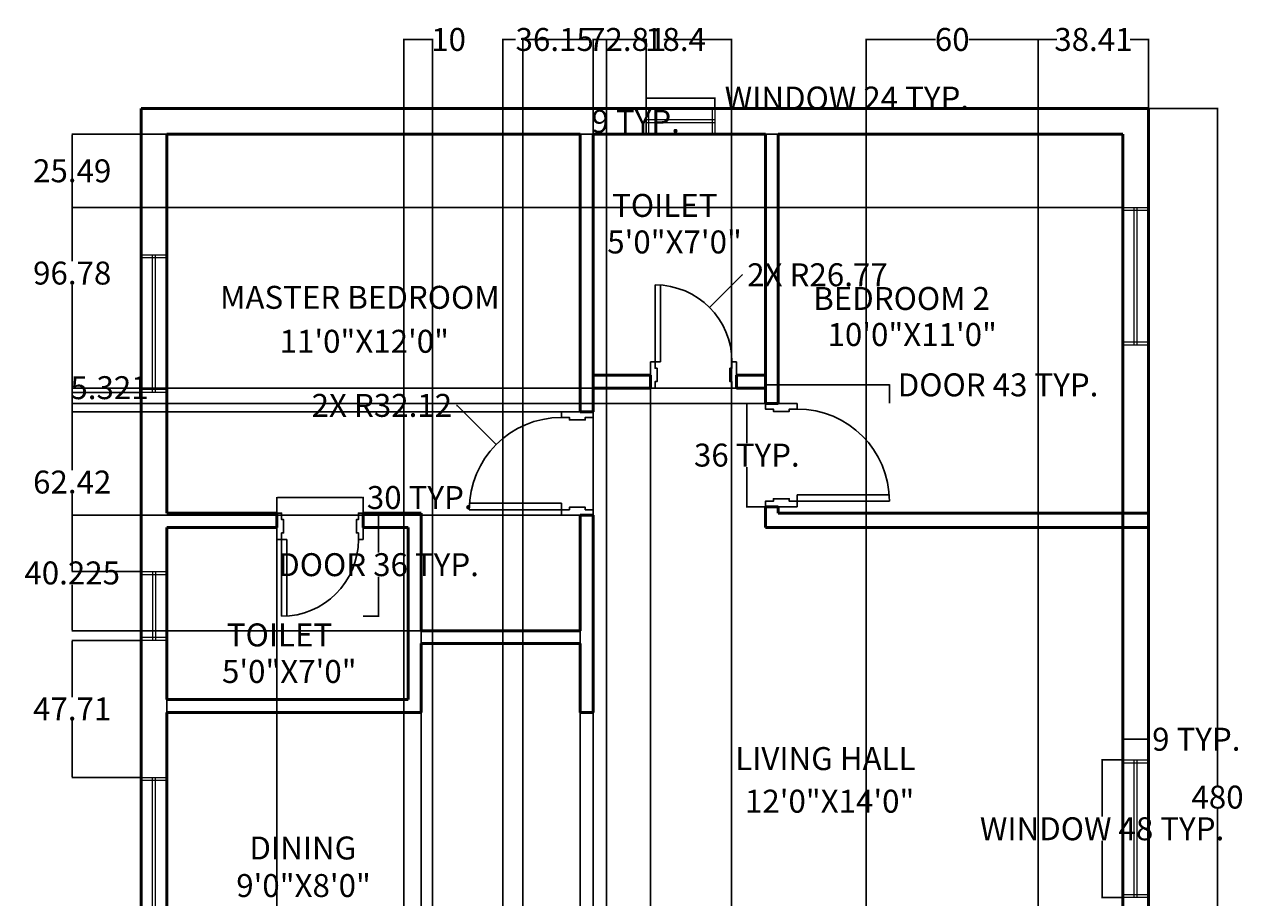
# Model space of a CAD drawing. Units: inches. Extents: x 16123781 to 16124206, y 158262361 to 158262900.
# Tile 2 of 2: x 16123781 to 16124206, y 158262596 to 158262900. Entities that reach past the tile are written whole.
import ezdxf

# ---------------------------------------------------------------- set-up
doc = ezdxf.new("R2010")
doc.units = ezdxf.units.IN
for name, color, linetype, lineweight in [('A-ANNO-DIMS', 2, 'Continuous', 18), ('A-AREA-IDEN', 7, 'Continuous', 25), ('A-Door', 150, 'Continuous', 25), ('wall', 130, 'Continuous', 50), ('window', 80, 'Continuous', 18)]:
    doc.layers.add(name, color=color, linetype=linetype, lineweight=lineweight)
doc.styles.get("Standard").update_dxf_attribs({"font": 'arial.ttf', "height": 8})
doc.dimstyles.get("Standard").update_dxf_attribs({"dimtxt": 0.18, "dimasz": 0.18, "dimexe": 0.18, "dimexo": 0.0625, "dimgap": 0.09, "dimtad": 0, "dimtih": 1, "dimtoh": 1, "dimdec": 4, "dimzin": 0, "dimdsep": 46, "dimtxsty": 'Standard', "dimcen": 0.09, "dimadec": 0, "dimazin": 0, "dimtfac": 1, "dimtdec": 4, "dimtofl": 0, "dimtmove": 0, "dimatfit": 3, "dimfxl": 1, "dimtolj": 1, "dimtzin": 0, "dimarcsym": 0})

# ---------------------------------------------------------------- blocks, each defined once
blk = doc.blocks.new('AP0B01')
blk.add_line((75, 100), (75, 678.7))
blk.add_lwpolyline([(35, 100), (35, 680, -0.449922)], format="xyb")
for points in [[(0, 100), (0, -100), (35, -100), (35, -50), (50, -50), (50, 50), (35, 50), (35, 100)], [(650, 100), (650, -100), (615, -100), (615, -50), (600, -50), (600, 50), (615, 50), (615, 100)]]:
    blk.add_lwpolyline(points, close=True)
blk.add_lwpolyline([(35, 100), (75, 100)])
blk.add_arc((35, 100), 580, 0, 90)
blk = doc.blocks.new('WIN-48IN')
for p, q in [((0, 0), (0, 48)), ((0, 48), (9, 48)), ((0, 47), (9, 47)), ((4, 0), (4, 48)), ((5, 0), (5, 48)), ((9, 48), (9, 0)), ((9, 1), (0, 1)), ((9, 0), (0, 0))]:
    blk.add_line(p, q)
blk = doc.blocks.new('WIN-24IN')
for p, q in [((0, 9), (24, 9)), ((0, 0), (0, 9)), ((1, 0), (1, 9)), ((23, 9), (23, 0)), ((24, 9), (24, 0)), ((24, 5), (0, 5)), ((24, 4), (0, 4)), ((24, 0), (0, 0))]:
    blk.add_line(p, q)
blk = doc.blocks.new('*D7')
at = {"layer": 'A-ANNO-DIMS', "color": 0, "lineweight": -2, "transparency": 16777216}
for p, q in [((16123899.14, 158262729.56), (16123904.65, 158262729.56)), ((16123904.47, 158262729.38), (16123904.47, 158262715.79)), ((16123904.47, 158262693.74), (16123904.47, 158262707.33)), ((16123899.14, 158262693.56), (16123904.65, 158262693.56))]:
    blk.add_line(p, q, dxfattribs=at)
at = {"layer": 'A-ANNO-DIMS', "color": 0, "transparency": 16777216}
for points in [[(16123904.44, 158262729.38), (16123904.5, 158262729.38), (16123904.47, 158262729.56)], [(16123904.44, 158262693.74), (16123904.5, 158262693.74), (16123904.47, 158262693.56)]]:
    blk.add_solid(points, dxfattribs=at)
at = {"layer": 'Defpoints', "color": 0, "transparency": 16777216}
for p in [(16123899.07, 158262729.56), (16123899.07, 158262693.56), (16123904.47, 158262693.56)]:
    blk.add_point(p, dxfattribs=at)
at = {"layer": 'A-ANNO-DIMS', "color": 0, "transparency": 16777216, "insert": (16123904.47, 158262711.56), "char_height": 8, "attachment_point": 5}
blk.add_mtext('\\A1;DOOR 36 TYP.', dxfattribs=at)
blk = doc.blocks.new('*D8')
at = {"layer": 'A-ANNO-DIMS', "color": 0, "lineweight": -2, "transparency": 16777216}
for p, q in [((16123869.07, 158262729.63), (16123869.07, 158262735.14)), ((16123869.25, 158262734.96), (16123898.89, 158262734.96)), ((16123899.07, 158262729.63), (16123899.07, 158262735.14)), ((16123899.07, 158262734.96), (16123899.25, 158262734.96))]:
    blk.add_line(p, q, dxfattribs=at)
at = {"layer": 'A-ANNO-DIMS', "color": 0, "transparency": 16777216}
for points in [[(16123869.25, 158262734.99), (16123869.25, 158262734.93), (16123869.07, 158262734.96)], [(16123898.89, 158262734.99), (16123898.89, 158262734.93), (16123899.07, 158262734.96)]]:
    blk.add_solid(points, dxfattribs=at)
at = {"layer": 'Defpoints', "color": 0, "transparency": 16777216}
for p in [(16123899.07, 158262734.96), (16123869.07, 158262729.56), (16123899.07, 158262729.56)]:
    blk.add_point(p, dxfattribs=at)
at = {"layer": 'A-ANNO-DIMS', "color": 0, "transparency": 16777216, "insert": (16123918.81, 158262734.96), "char_height": 8, "attachment_point": 5}
blk.add_mtext('\\A1;30 TYP.', dxfattribs=at)
blk = doc.blocks.new('*D9')
at = {"layer": 'A-ANNO-DIMS', "color": 0, "lineweight": -2, "transparency": 16777216}
for p, q in [((16124039.26, 158262767.8), (16124039.26, 158262774.4)), ((16124082.46, 158262767.8), (16124082.46, 158262774.4)), ((16124039.44, 158262774.22), (16124082.28, 158262774.22)), ((16124082.46, 158262774.22), (16124082.64, 158262774.22))]:
    blk.add_line(p, q, dxfattribs=at)
at = {"layer": 'A-ANNO-DIMS', "color": 0, "transparency": 16777216}
for points in [[(16124039.44, 158262774.25), (16124039.44, 158262774.19), (16124039.26, 158262774.22)], [(16124082.28, 158262774.25), (16124082.28, 158262774.19), (16124082.46, 158262774.22)]]:
    blk.add_solid(points, dxfattribs=at)
at = {"layer": 'Defpoints', "color": 0, "transparency": 16777216}
for p in [(16124082.46, 158262774.22), (16124039.26, 158262767.74), (16124082.46, 158262767.74)]:
    blk.add_point(p, dxfattribs=at)
at = {"layer": 'A-ANNO-DIMS', "color": 0, "transparency": 16777216, "insert": (16124120.32, 158262774.22), "char_height": 8, "attachment_point": 5}
blk.add_mtext('\\A1;DOOR 43 TYP.', dxfattribs=at)
blk = doc.blocks.new('*D10')
at = {"layer": 'A-ANNO-DIMS', "color": 0, "lineweight": -2, "transparency": 16777216}
for p, q in [((16124039.2, 158262767.74), (16124032.6, 158262767.74)), ((16124032.78, 158262767.56), (16124032.78, 158262753.92)), ((16124032.78, 158262731.92), (16124032.78, 158262745.56)), ((16124039.2, 158262731.74), (16124032.6, 158262731.74))]:
    blk.add_line(p, q, dxfattribs=at)
at = {"layer": 'A-ANNO-DIMS', "color": 0, "transparency": 16777216}
for points in [[(16124032.75, 158262767.56), (16124032.81, 158262767.56), (16124032.78, 158262767.74)], [(16124032.75, 158262731.92), (16124032.81, 158262731.92), (16124032.78, 158262731.74)]]:
    blk.add_solid(points, dxfattribs=at)
at = {"layer": 'Defpoints', "color": 0, "transparency": 16777216}
for p in [(16124032.78, 158262767.74), (16124039.26, 158262767.74), (16124039.26, 158262731.74)]:
    blk.add_point(p, dxfattribs=at)
at = {"layer": 'A-ANNO-DIMS', "color": 0, "transparency": 16777216, "insert": (16124032.78, 158262749.74), "char_height": 8, "attachment_point": 5}
blk.add_mtext('\\A1;36 TYP.', dxfattribs=at)
blk = doc.blocks.new('*D11')
at = {"layer": 'A-ANNO-DIMS', "color": 0, "lineweight": -2, "transparency": 16777216}
for p, q in [((16124163.7, 158262643.53), (16124156.38, 158262643.53)), ((16124156.56, 158262643.35), (16124156.56, 158262623.76)), ((16124156.56, 158262595.71), (16124156.56, 158262615.31)), ((16124163.7, 158262595.53), (16124156.38, 158262595.53))]:
    blk.add_line(p, q, dxfattribs=at)
at = {"layer": 'A-ANNO-DIMS', "color": 0, "transparency": 16777216}
for points in [[(16124156.53, 158262643.35), (16124156.59, 158262643.35), (16124156.56, 158262643.53)], [(16124156.53, 158262595.71), (16124156.59, 158262595.71), (16124156.56, 158262595.53)]]:
    blk.add_solid(points, dxfattribs=at)
at = {"layer": 'Defpoints', "color": 0, "transparency": 16777216}
for p in [(16124156.56, 158262643.53), (16124163.76, 158262643.53), (16124163.76, 158262595.53)]:
    blk.add_point(p, dxfattribs=at)
at = {"layer": 'A-ANNO-DIMS', "color": 0, "transparency": 16777216, "insert": (16124156.56, 158262619.53), "char_height": 8, "attachment_point": 5}
blk.add_mtext('\\A1;WINDOW 48 TYP.', dxfattribs=at)
blk = doc.blocks.new('*D12')
at = {"layer": 'A-ANNO-DIMS', "color": 0, "lineweight": -2, "transparency": 16777216}
for p, q in [((16124163.76, 158262643.6), (16124163.76, 158262650.91)), ((16124163.94, 158262650.73), (16124172.58, 158262650.73)), ((16124172.76, 158262643.6), (16124172.76, 158262650.91)), ((16124172.76, 158262650.73), (16124172.94, 158262650.73))]:
    blk.add_line(p, q, dxfattribs=at)
at = {"layer": 'A-ANNO-DIMS', "color": 0, "transparency": 16777216}
for points in [[(16124163.94, 158262650.76), (16124163.94, 158262650.7), (16124163.76, 158262650.73)], [(16124172.58, 158262650.76), (16124172.58, 158262650.7), (16124172.76, 158262650.73)]]:
    blk.add_solid(points, dxfattribs=at)
at = {"layer": 'Defpoints', "color": 0, "transparency": 16777216}
for p in [(16124172.76, 158262650.73), (16124163.76, 158262643.53), (16124172.76, 158262643.53)]:
    blk.add_point(p, dxfattribs=at)
at = {"layer": 'A-ANNO-DIMS', "color": 0, "transparency": 16777216, "insert": (16124189.39, 158262650.73), "char_height": 8, "attachment_point": 5}
blk.add_mtext('\\A1;9 TYP.', dxfattribs=at)
blk = doc.blocks.new('*D13')
at = {"layer": 'A-ANNO-DIMS', "color": 0, "lineweight": -2, "transparency": 16777216}
for p, q in [((16123997.66, 158262870.63), (16123997.66, 158262874.34)), ((16123997.84, 158262874.16), (16124021.48, 158262874.16)), ((16124021.66, 158262870.63), (16124021.66, 158262874.34)), ((16124021.66, 158262874.16), (16124021.84, 158262874.16))]:
    blk.add_line(p, q, dxfattribs=at)
at = {"layer": 'A-ANNO-DIMS', "color": 0, "transparency": 16777216}
for points in [[(16123997.84, 158262874.19), (16123997.84, 158262874.13), (16123997.66, 158262874.16)], [(16124021.48, 158262874.19), (16124021.48, 158262874.13), (16124021.66, 158262874.16)]]:
    blk.add_solid(points, dxfattribs=at)
at = {"layer": 'Defpoints', "color": 0, "transparency": 16777216}
for p in [(16124021.66, 158262874.16), (16123997.66, 158262870.56), (16124021.66, 158262870.56)]:
    blk.add_point(p, dxfattribs=at)
at = {"layer": 'A-ANNO-DIMS', "color": 0, "transparency": 16777216, "insert": (16124067.64, 158262874.16), "char_height": 8, "attachment_point": 5}
blk.add_mtext('\\A1;WINDOW 24 TYP.', dxfattribs=at)
blk = doc.blocks.new('*D14')
at = {"layer": 'A-ANNO-DIMS', "color": 0, "lineweight": -2, "transparency": 16777216}
for p, q in [((16123997.6, 158262870.56), (16123993.88, 158262870.56)), ((16123994.06, 158262870.38), (16123994.06, 158262870.24)), ((16123997.6, 158262861.56), (16123993.88, 158262861.56)), ((16123994.06, 158262861.74), (16123994.06, 158262861.89))]:
    blk.add_line(p, q, dxfattribs=at)
at = {"layer": 'A-ANNO-DIMS', "color": 0, "transparency": 16777216}
for points in [[(16123994.03, 158262870.38), (16123994.09, 158262870.38), (16123994.06, 158262870.56)], [(16123994.03, 158262861.74), (16123994.09, 158262861.74), (16123994.06, 158262861.56)]]:
    blk.add_solid(points, dxfattribs=at)
at = {"layer": 'Defpoints', "color": 0, "transparency": 16777216}
for p in [(16123994.06, 158262870.56), (16123997.66, 158262870.56), (16123997.66, 158262861.56)]:
    blk.add_point(p, dxfattribs=at)
at = {"layer": 'A-ANNO-DIMS', "color": 0, "transparency": 16777216, "insert": (16123994.06, 158262866.06), "char_height": 8, "attachment_point": 5}
blk.add_mtext('\\A1;9 TYP.', dxfattribs=at)
blk = doc.blocks.new('*D18')
at = {"layer": 'A-ANNO-DIMS', "color": 0, "lineweight": -2, "transparency": 16777216}
for p, q in [((16124172.82, 158262870.56), (16124196.97, 158262870.56)), ((16124196.79, 158262870.38), (16124196.79, 158262634.74)), ((16124196.79, 158262390.74), (16124196.79, 158262626.39)), ((16124172.82, 158262390.56), (16124196.97, 158262390.56))]:
    blk.add_line(p, q, dxfattribs=at)
at = {"layer": 'A-ANNO-DIMS', "color": 0, "transparency": 16777216}
for points in [[(16124196.76, 158262870.38), (16124196.82, 158262870.38), (16124196.79, 158262870.56)], [(16124196.76, 158262390.74), (16124196.82, 158262390.74), (16124196.79, 158262390.56)]]:
    blk.add_solid(points, dxfattribs=at)
at = {"layer": 'Defpoints', "color": 0, "transparency": 16777216}
for p in [(16124172.76, 158262870.56), (16124196.79, 158262870.56), (16124172.76, 158262390.56)]:
    blk.add_point(p, dxfattribs=at)
at = {"layer": 'A-ANNO-DIMS', "color": 0, "transparency": 16777216, "insert": (16124196.79, 158262630.56), "char_height": 8, "attachment_point": 5}
blk.add_mtext('\\A1;480', dxfattribs=at)
blk = doc.blocks.new('*D19')
at = {"layer": 'A-ANNO-DIMS', "color": 0, "lineweight": -2, "transparency": 16777216}
for p, q in [((16124074.35, 158262390.63), (16124074.35, 158262894.77)), ((16124074.53, 158262894.59), (16124098.52, 158262894.59)), ((16124134.17, 158262894.59), (16124110.18, 158262894.59)), ((16124134.35, 158262390.63), (16124134.35, 158262894.77))]:
    blk.add_line(p, q, dxfattribs=at)
at = {"layer": 'A-ANNO-DIMS', "color": 0, "transparency": 16777216}
for points in [[(16124074.53, 158262894.62), (16124074.53, 158262894.56), (16124074.35, 158262894.59)], [(16124134.17, 158262894.62), (16124134.17, 158262894.56), (16124134.35, 158262894.59)]]:
    blk.add_solid(points, dxfattribs=at)
at = {"layer": 'Defpoints', "color": 0, "transparency": 16777216}
for p in [(16124134.35, 158262894.59), (16124074.35, 158262390.56), (16124134.35, 158262390.56)]:
    blk.add_point(p, dxfattribs=at)
at = {"layer": 'A-ANNO-DIMS', "color": 0, "transparency": 16777216, "insert": (16124104.35, 158262894.59), "char_height": 8, "attachment_point": 5}
blk.add_mtext('\\A1;60', dxfattribs=at)
blk = doc.blocks.new('*D20')
at = {"layer": 'A-ANNO-DIMS', "color": 0, "lineweight": -2, "transparency": 16777216}
for p, q in [((16124134.35, 158262390.63), (16124134.35, 158262894.77)), ((16124134.53, 158262894.59), (16124140.74, 158262894.59)), ((16124172.58, 158262894.59), (16124166.37, 158262894.59)), ((16124172.76, 158262390.63), (16124172.76, 158262894.77))]:
    blk.add_line(p, q, dxfattribs=at)
at = {"layer": 'A-ANNO-DIMS', "color": 0, "transparency": 16777216}
for points in [[(16124134.53, 158262894.62), (16124134.53, 158262894.56), (16124134.35, 158262894.59)], [(16124172.58, 158262894.62), (16124172.58, 158262894.56), (16124172.76, 158262894.59)]]:
    blk.add_solid(points, dxfattribs=at)
at = {"layer": 'Defpoints', "color": 0, "transparency": 16777216}
for p in [(16124172.76, 158262894.59), (16124134.35, 158262390.56), (16124172.76, 158262390.56)]:
    blk.add_point(p, dxfattribs=at)
at = {"layer": 'A-ANNO-DIMS', "color": 0, "transparency": 16777216, "insert": (16124153.55, 158262894.59), "char_height": 8, "attachment_point": 5}
blk.add_mtext('\\A1;38.41', dxfattribs=at)
blk = doc.blocks.new('*D23')
at = {"layer": 'A-ANNO-DIMS', "color": 0, "lineweight": -2, "transparency": 16777216}
for p, q in [((16123947.76, 158262503.13), (16123947.76, 158262894.77)), ((16123947.94, 158262894.59), (16123952.22, 158262894.59)), ((16123983.73, 158262894.59), (16123979.45, 158262894.59)), ((16123983.91, 158262503.13), (16123983.91, 158262894.77))]:
    blk.add_line(p, q, dxfattribs=at)
at = {"layer": 'A-ANNO-DIMS', "color": 0, "transparency": 16777216}
for points in [[(16123947.94, 158262894.62), (16123947.94, 158262894.56), (16123947.76, 158262894.59)], [(16123983.73, 158262894.62), (16123983.73, 158262894.56), (16123983.91, 158262894.59)]]:
    blk.add_solid(points, dxfattribs=at)
at = {"layer": 'Defpoints', "color": 0, "transparency": 16777216}
for p in [(16123983.91, 158262894.59), (16123947.76, 158262503.06), (16123983.91, 158262503.06)]:
    blk.add_point(p, dxfattribs=at)
at = {"layer": 'A-ANNO-DIMS', "color": 0, "transparency": 16777216, "insert": (16123965.84, 158262894.59), "char_height": 8, "attachment_point": 5}
blk.add_mtext('\\A1;36.15', dxfattribs=at)
blk = doc.blocks.new('*D29')
at = {"layer": 'A-ANNO-DIMS', "color": 0, "lineweight": -2, "transparency": 16777216}
for p, q in [((16123821.7, 158262685.14), (16123797.55, 158262685.14)), ((16123797.73, 158262684.96), (16123797.73, 158262665.39)), ((16123797.73, 158262637.61), (16123797.73, 158262657.18)), ((16123821.7, 158262637.43), (16123797.55, 158262637.43))]:
    blk.add_line(p, q, dxfattribs=at)
at = {"layer": 'A-ANNO-DIMS', "color": 0, "transparency": 16777216}
for points in [[(16123797.7, 158262684.96), (16123797.76, 158262684.96), (16123797.73, 158262685.14)], [(16123797.7, 158262637.61), (16123797.76, 158262637.61), (16123797.73, 158262637.43)]]:
    blk.add_solid(points, dxfattribs=at)
at = {"layer": 'Defpoints', "color": 0, "transparency": 16777216}
for p in [(16123797.73, 158262685.14), (16123821.76, 158262685.14), (16123821.76, 158262637.43)]:
    blk.add_point(p, dxfattribs=at)
at = {"layer": 'A-ANNO-DIMS', "color": 0, "transparency": 16777216, "insert": (16123797.73, 158262661.29), "char_height": 8, "attachment_point": 5}
blk.add_mtext('\\A1;47.71', dxfattribs=at)
blk = doc.blocks.new('*D30')
at = {"layer": 'A-ANNO-DIMS', "color": 0, "lineweight": -2, "transparency": 16777216}
for p, q in [((16123821.7, 158262771.56), (16123797.55, 158262771.56)), ((16123797.73, 158262771.38), (16123797.73, 158262744.53)), ((16123797.73, 158262709.32), (16123797.73, 158262736.18)), ((16123821.7, 158262709.14), (16123797.55, 158262709.14))]:
    blk.add_line(p, q, dxfattribs=at)
at = {"layer": 'A-ANNO-DIMS', "color": 0, "transparency": 16777216}
for points in [[(16123797.7, 158262771.38), (16123797.76, 158262771.38), (16123797.73, 158262771.56)], [(16123797.7, 158262709.32), (16123797.76, 158262709.32), (16123797.73, 158262709.14)]]:
    blk.add_solid(points, dxfattribs=at)
at = {"layer": 'Defpoints', "color": 0, "transparency": 16777216}
for p in [(16123797.73, 158262771.56), (16123821.76, 158262771.56), (16123821.76, 158262709.14)]:
    blk.add_point(p, dxfattribs=at)
at = {"layer": 'A-ANNO-DIMS', "color": 0, "transparency": 16777216, "insert": (16123797.73, 158262740.35), "char_height": 8, "attachment_point": 5}
blk.add_mtext('\\A1;62.42', dxfattribs=at)
blk = doc.blocks.new('*D32')
at = {"layer": 'A-ANNO-DIMS', "color": 0, "lineweight": -2, "transparency": 16777216}
for p, q in [((16124163.7, 158262861.56), (16123797.55, 158262861.56)), ((16123797.73, 158262861.38), (16123797.73, 158262852.99)), ((16123797.73, 158262836.25), (16123797.73, 158262844.64)), ((16124163.7, 158262836.07), (16123797.55, 158262836.07))]:
    blk.add_line(p, q, dxfattribs=at)
at = {"layer": 'A-ANNO-DIMS', "color": 0, "transparency": 16777216}
for points in [[(16123797.7, 158262861.38), (16123797.76, 158262861.38), (16123797.73, 158262861.56)], [(16123797.7, 158262836.25), (16123797.76, 158262836.25), (16123797.73, 158262836.07)]]:
    blk.add_solid(points, dxfattribs=at)
at = {"layer": 'Defpoints', "color": 0, "transparency": 16777216}
for p in [(16123797.73, 158262861.56), (16124163.76, 158262861.56), (16124163.76, 158262836.07)]:
    blk.add_point(p, dxfattribs=at)
at = {"layer": 'A-ANNO-DIMS', "color": 0, "transparency": 16777216, "insert": (16123797.73, 158262848.82), "char_height": 8, "attachment_point": 5}
blk.add_mtext('\\A1;25.49', dxfattribs=at)
blk = doc.blocks.new('*D33')
at = {"layer": 'A-ANNO-DIMS', "color": 0, "lineweight": -2, "transparency": 16777216}
for p, q in [((16123979.26, 158262861.63), (16123979.26, 158262894.77)), ((16123979.44, 158262894.59), (16123997.48, 158262894.59)), ((16123997.66, 158262861.63), (16123997.66, 158262894.77)), ((16123997.66, 158262894.59), (16123997.84, 158262894.59))]:
    blk.add_line(p, q, dxfattribs=at)
at = {"layer": 'A-ANNO-DIMS', "color": 0, "transparency": 16777216}
for points in [[(16123979.44, 158262894.62), (16123979.44, 158262894.56), (16123979.26, 158262894.59)], [(16123997.48, 158262894.62), (16123997.48, 158262894.56), (16123997.66, 158262894.59)]]:
    blk.add_solid(points, dxfattribs=at)
at = {"layer": 'Defpoints', "color": 0, "transparency": 16777216}
for p in [(16123997.66, 158262894.59), (16123979.26, 158262861.56), (16123997.66, 158262861.56)]:
    blk.add_point(p, dxfattribs=at)
at = {"layer": 'A-ANNO-DIMS', "color": 0, "transparency": 16777216, "insert": (16124007.93, 158262894.59), "char_height": 8, "attachment_point": 5}
blk.add_mtext('\\A1;18.4', dxfattribs=at)
blk = doc.blocks.new('*D35')
at = {"layer": 'A-ANNO-DIMS', "color": 0, "lineweight": -2, "transparency": 16777216}
for p, q in [((16123913.26, 158262484.13), (16123913.26, 158262894.77)), ((16123913.44, 158262894.59), (16123923.08, 158262894.59)), ((16123923.26, 158262484.13), (16123923.26, 158262894.77)), ((16123923.26, 158262894.59), (16123923.44, 158262894.59))]:
    blk.add_line(p, q, dxfattribs=at)
at = {"layer": 'A-ANNO-DIMS', "color": 0, "transparency": 16777216}
for points in [[(16123913.44, 158262894.62), (16123913.44, 158262894.56), (16123913.26, 158262894.59)], [(16123923.08, 158262894.62), (16123923.08, 158262894.56), (16123923.26, 158262894.59)]]:
    blk.add_solid(points, dxfattribs=at)
at = {"layer": 'Defpoints', "color": 0, "transparency": 16777216}
for p in [(16123923.26, 158262894.59), (16123913.26, 158262484.06), (16123923.26, 158262484.06)]:
    blk.add_point(p, dxfattribs=at)
at = {"layer": 'A-ANNO-DIMS', "color": 0, "transparency": 16777216, "insert": (16123928.87, 158262894.59), "char_height": 8, "attachment_point": 5}
blk.add_mtext('\\A1;10', dxfattribs=at)
blk = doc.blocks.new('*D36')
at = {"layer": 'A-ANNO-DIMS', "color": 0, "lineweight": -2, "transparency": 16777216}
for p, q in [((16123954.69, 158262552.13), (16123954.69, 158262894.77)), ((16123954.87, 158262894.59), (16123978.31, 158262894.59)), ((16124027.32, 158262894.59), (16124003.88, 158262894.59)), ((16124027.5, 158262552.13), (16124027.5, 158262894.77))]:
    blk.add_line(p, q, dxfattribs=at)
at = {"layer": 'A-ANNO-DIMS', "color": 0, "transparency": 16777216}
for points in [[(16123954.87, 158262894.62), (16123954.87, 158262894.56), (16123954.69, 158262894.59)], [(16124027.32, 158262894.62), (16124027.32, 158262894.56), (16124027.5, 158262894.59)]]:
    blk.add_solid(points, dxfattribs=at)
at = {"layer": 'Defpoints', "color": 0, "transparency": 16777216}
for p in [(16124027.5, 158262894.59), (16123954.69, 158262552.06), (16124027.5, 158262552.06)]:
    blk.add_point(p, dxfattribs=at)
at = {"layer": 'A-ANNO-DIMS', "color": 0, "transparency": 16777216, "insert": (16123991.1, 158262894.59), "char_height": 8, "attachment_point": 5}
blk.add_mtext('\\A1;72.81', dxfattribs=at)
blk = doc.blocks.new('*D37')
at = {"layer": 'A-ANNO-DIMS', "color": 0, "lineweight": -2, "transparency": 16777216}
for p, q in [((16123919.260748, 158262688.500323), (16123919.260748, 158262366.352823)), ((16123974.760748, 158262688.500323), (16123974.760748, 158262366.352823)), ((16123919.440748, 158262366.532823), (16123936.500557, 158262366.532823)), ((16123974.580748, 158262366.532823), (16123957.520939, 158262366.532823))]:
    blk.add_line(p, q, dxfattribs=at)
at = {"layer": 'A-ANNO-DIMS', "color": 0, "transparency": 16777216}
for points in [[(16123919.440748, 158262366.562823), (16123919.440748, 158262366.502823), (16123919.260748, 158262366.532823)], [(16123974.580748, 158262366.562823), (16123974.580748, 158262366.502823), (16123974.760748, 158262366.532823)]]:
    blk.add_solid(points, dxfattribs=at)
at = {"layer": 'Defpoints', "color": 0, "transparency": 16777216}
for p in [(16123919.260748, 158262688.562823), (16123974.760748, 158262688.562823), (16123974.760748, 158262366.532823)]:
    blk.add_point(p, dxfattribs=at)
at = {"layer": 'A-ANNO-DIMS', "color": 0, "transparency": 16777216, "insert": (16123947.010748, 158262366.532823), "char_height": 8, "attachment_point": 5}
blk.add_mtext('\\A1;55.5', dxfattribs=at)
blk = doc.blocks.new('*D38')
at = {"layer": 'A-ANNO-DIMS', "color": 0, "lineweight": -2, "transparency": 16777216}
for p, q in [((16123974.7, 158262728.79), (16123797.55, 158262728.79)), ((16123797.73, 158262728.61), (16123797.73, 158262712.85)), ((16123797.73, 158262688.74), (16123797.73, 158262704.5)), ((16123974.7, 158262688.56), (16123797.55, 158262688.56))]:
    blk.add_line(p, q, dxfattribs=at)
at = {"layer": 'A-ANNO-DIMS', "color": 0, "transparency": 16777216}
for points in [[(16123797.7, 158262728.61), (16123797.76, 158262728.61), (16123797.73, 158262728.79)], [(16123797.7, 158262688.74), (16123797.76, 158262688.74), (16123797.73, 158262688.56)]]:
    blk.add_solid(points, dxfattribs=at)
at = {"layer": 'Defpoints', "color": 0, "transparency": 16777216}
for p in [(16123797.73, 158262728.79), (16123974.76, 158262728.79), (16123974.76, 158262688.56)]:
    blk.add_point(p, dxfattribs=at)
at = {"layer": 'A-ANNO-DIMS', "color": 0, "transparency": 16777216, "insert": (16123797.73, 158262708.68), "char_height": 8, "attachment_point": 5}
blk.add_mtext('\\A1;40.225', dxfattribs=at)
blk = doc.blocks.new('*D39')
at = {"layer": 'A-ANNO-DIMS', "color": 0, "lineweight": -2, "transparency": 16777216}
for p, q in [((16123974.760748, 158262660.000323), (16123974.760748, 158262366.352823)), ((16123979.260748, 158262660.000323), (16123979.260748, 158262366.352823)), ((16123974.940748, 158262366.532823), (16123979.080748, 158262366.532823)), ((16123979.260748, 158262366.532823), (16123979.440748, 158262366.532823))]:
    blk.add_line(p, q, dxfattribs=at)
at = {"layer": 'A-ANNO-DIMS', "color": 0, "transparency": 16777216}
for points in [[(16123974.940748, 158262366.562823), (16123974.940748, 158262366.502823), (16123974.760748, 158262366.532823)], [(16123979.080748, 158262366.562823), (16123979.080748, 158262366.502823), (16123979.260748, 158262366.532823)]]:
    blk.add_solid(points, dxfattribs=at)
at = {"layer": 'Defpoints', "color": 0, "transparency": 16777216}
for p in [(16123974.760748, 158262660.062823), (16123979.260748, 158262660.062823), (16123979.260748, 158262366.532823)]:
    blk.add_point(p, dxfattribs=at)
at = {"layer": 'A-ANNO-DIMS', "color": 0, "transparency": 16777216, "insert": (16123987.004145, 158262366.532823), "char_height": 8, "attachment_point": 5}
blk.add_mtext('\\A1;4.5', dxfattribs=at)
blk = doc.blocks.new('*D40')
at = {"layer": 'A-ANNO-DIMS', "color": 0, "lineweight": -2, "transparency": 16777216}
for p, q in [((16123830.76, 158262724.5), (16123830.76, 158262366.35)), ((16123869.07, 158262724.5), (16123869.07, 158262366.35)), ((16123830.94, 158262366.53), (16123837.1, 158262366.53)), ((16123868.89, 158262366.53), (16123862.73, 158262366.53))]:
    blk.add_line(p, q, dxfattribs=at)
at = {"layer": 'A-ANNO-DIMS', "color": 0, "transparency": 16777216}
for points in [[(16123830.94, 158262366.56), (16123830.94, 158262366.5), (16123830.76, 158262366.53)], [(16123868.89, 158262366.56), (16123868.89, 158262366.5), (16123869.07, 158262366.53)]]:
    blk.add_solid(points, dxfattribs=at)
at = {"layer": 'Defpoints', "color": 0, "transparency": 16777216}
for p in [(16123830.76, 158262724.56), (16123869.07, 158262724.56), (16123869.07, 158262366.53)]:
    blk.add_point(p, dxfattribs=at)
at = {"layer": 'A-ANNO-DIMS', "color": 0, "transparency": 16777216, "insert": (16123849.92, 158262366.53), "char_height": 8, "attachment_point": 5}
blk.add_mtext('\\A1;38.31', dxfattribs=at)
blk = doc.blocks.new('*D41')
at = {"layer": 'A-ANNO-DIMS', "color": 0, "lineweight": -2, "transparency": 16777216}
for p, q in [((16123979.26, 158262777.5), (16123979.26, 158262366.35)), ((16123999.23, 158262777.5), (16123999.23, 158262366.35)), ((16123979.44, 158262366.53), (16123999.05, 158262366.53)), ((16123999.23, 158262366.53), (16123999.41, 158262366.53))]:
    blk.add_line(p, q, dxfattribs=at)
at = {"layer": 'A-ANNO-DIMS', "color": 0, "transparency": 16777216}
for points in [[(16123979.44, 158262366.56), (16123979.44, 158262366.5), (16123979.26, 158262366.53)], [(16123999.05, 158262366.56), (16123999.05, 158262366.5), (16123999.23, 158262366.53)]]:
    blk.add_solid(points, dxfattribs=at)
at = {"layer": 'Defpoints', "color": 0, "transparency": 16777216}
for p in [(16123979.26, 158262777.56), (16123999.23, 158262777.56), (16123999.23, 158262366.53)]:
    blk.add_point(p, dxfattribs=at)
at = {"layer": 'A-ANNO-DIMS', "color": 0, "transparency": 16777216, "insert": (16124015.73, 158262366.53), "char_height": 8, "attachment_point": 5}
blk.add_mtext('\\A1;19.967', dxfattribs=at)
blk = doc.blocks.new('*D42')
at = {"layer": 'A-ANNO-DIMS', "color": 0, "lineweight": -2, "transparency": 16777216}
for p, q in [((16124039.2, 158262773.06), (16123797.55, 158262773.06)), ((16123797.73, 158262773.06), (16123797.73, 158262773.24)), ((16123797.73, 158262773.24), (16123797.91, 158262773.24)), ((16123797.73, 158262767.92), (16123797.73, 158262772.88)), ((16124039.2, 158262767.74), (16123797.55, 158262767.74))]:
    blk.add_line(p, q, dxfattribs=at)
at = {"layer": 'A-ANNO-DIMS', "color": 0, "transparency": 16777216}
for points in [[(16123797.7, 158262772.88), (16123797.76, 158262772.88), (16123797.73, 158262773.06)], [(16123797.7, 158262767.92), (16123797.76, 158262767.92), (16123797.73, 158262767.74)]]:
    blk.add_solid(points, dxfattribs=at)
at = {"layer": 'Defpoints', "color": 0, "transparency": 16777216}
for p in [(16123797.73, 158262773.06), (16124039.26, 158262773.06), (16124039.26, 158262767.74)]:
    blk.add_point(p, dxfattribs=at)
at = {"layer": 'A-ANNO-DIMS', "color": 0, "transparency": 16777216, "insert": (16123810.73, 158262773.24), "char_height": 8, "attachment_point": 5}
blk.add_mtext('\\A1;5.321', dxfattribs=at)
blk = doc.blocks.new('*D43')
at = {"layer": 'A-ANNO-DIMS', "color": 0, "lineweight": -2, "transparency": 16777216}
for p, q in [((16123974.7, 158262861.56), (16123797.55, 158262861.56)), ((16123797.73, 158262861.38), (16123797.73, 158262817.35)), ((16123797.73, 158262764.97), (16123797.73, 158262809)), ((16123974.7, 158262764.79), (16123797.55, 158262764.79))]:
    blk.add_line(p, q, dxfattribs=at)
at = {"layer": 'A-ANNO-DIMS', "color": 0, "transparency": 16777216}
for points in [[(16123797.7, 158262861.38), (16123797.76, 158262861.38), (16123797.73, 158262861.56)], [(16123797.7, 158262764.97), (16123797.76, 158262764.97), (16123797.73, 158262764.79)]]:
    blk.add_solid(points, dxfattribs=at)
at = {"layer": 'Defpoints', "color": 0, "transparency": 16777216}
for p in [(16123797.73, 158262861.56), (16123974.76, 158262861.56), (16123974.76, 158262764.79)]:
    blk.add_point(p, dxfattribs=at)
at = {"layer": 'A-ANNO-DIMS', "color": 0, "transparency": 16777216, "insert": (16123797.73, 158262813.18), "char_height": 8, "attachment_point": 5}
blk.add_mtext('\\A1;96.78', dxfattribs=at)
blk = doc.blocks.new('*D44')
at = {"layer": 'A-ANNO-DIMS', "color": 0, "lineweight": -2, "transparency": 16777216}
for p, q in [((16123931.66, 158262767.07), (16123931.84, 158262767.07)), ((16123931.84, 158262767.07), (16123945.34, 158262753.57)), ((16123968.09, 158262730.73), (16123968.27, 158262730.73)), ((16123968.18, 158262730.64), (16123968.18, 158262730.82))]:
    blk.add_line(p, q, dxfattribs=at)
at = {"layer": 'A-ANNO-DIMS', "color": 0, "transparency": 16777216}
blk.add_solid([(16123945.36, 158262753.59), (16123945.32, 158262753.55), (16123945.47, 158262753.44)], dxfattribs=at)
at = {"layer": 'Defpoints', "color": 0, "transparency": 16777216}
for p in [(16123945.47, 158262753.44), (16123968.18, 158262730.73)]:
    blk.add_point(p, dxfattribs=at)
at = {"layer": 'A-ANNO-DIMS', "color": 0, "transparency": 16777216, "insert": (16123905.62, 158262767.07), "char_height": 8, "attachment_point": 5}
blk.add_mtext('\\A1;2X R32.12', dxfattribs=at)
blk = doc.blocks.new('*D45')
at = {"layer": 'A-ANNO-DIMS', "color": 0, "lineweight": -2, "transparency": 16777216}
for p, q in [((16124031.13, 158262812.58), (16124019.9, 158262801.35)), ((16124031.31, 158262812.58), (16124031.13, 158262812.58)), ((16124000.75, 158262782.29), (16124000.93, 158262782.29)), ((16124000.84, 158262782.2), (16124000.84, 158262782.38))]:
    blk.add_line(p, q, dxfattribs=at)
at = {"layer": 'A-ANNO-DIMS', "color": 0, "transparency": 16777216}
blk.add_solid([(16124019.88, 158262801.37), (16124019.92, 158262801.33), (16124019.77, 158262801.22)], dxfattribs=at)
at = {"layer": 'Defpoints', "color": 0, "transparency": 16777216}
for p in [(16124019.77, 158262801.22), (16124000.84, 158262782.29)]:
    blk.add_point(p, dxfattribs=at)
at = {"layer": 'A-ANNO-DIMS', "color": 0, "transparency": 16777216, "insert": (16124057.39, 158262812.58), "char_height": 8, "attachment_point": 5}
blk.add_mtext('\\A1;2X R26.77', dxfattribs=at)

msp = doc.modelspace()

# ---------------------------------------------------------------- linework, layer by layer
at = {"layer": 'wall'}
for p, q in [((16123821.7607, 158262870.5628), (16123821.7607, 158262390.5628)), ((16123821.7607, 158262870.5628), (16124172.7607, 158262870.5628)), ((16124172.7607, 158262870.5628), (16124172.7607, 158262390.5628)), ((16123830.7607, 158262861.5628), (16123974.7607, 158262861.5628)), ((16123830.7607, 158262861.5628), (16123830.7607, 158262729.5628)), ((16123974.7607, 158262861.5628), (16123974.7607, 158262764.7877)), ((16123979.2607, 158262861.5628), (16124039.2607, 158262861.5628)), ((16123979.2607, 158262861.5628), (16123979.2607, 158262764.7877)), ((16124039.2607, 158262861.5628), (16124039.2607, 158262767.742)), ((16124043.7607, 158262861.5628), (16124163.7607, 158262861.5628)), ((16124043.7607, 158262861.5628), (16124043.7607, 158262767.742)), ((16124163.7607, 158262861.5628), (16124163.7607, 158262556.5628)), ((16123979.2607, 158262777.5628), (16123999.2273, 158262777.5628)), ((16123999.2273, 158262777.5628), (16123999.2273, 158262773.0628)), ((16124029.2273, 158262777.5628), (16124029.2273, 158262773.0628)), ((16124029.2273, 158262777.5628), (16124039.2607, 158262777.5628)), ((16123979.2607, 158262773.0628), (16123999.2273, 158262773.0628)), ((16124029.2273, 158262773.0628), (16124039.2607, 158262773.0628)), ((16124043.7607, 158262767.742), (16124039.2607, 158262767.742)), ((16123979.2607, 158262764.7877), (16123974.7607, 158262764.7877)), ((16123830.7607, 158262729.5628), (16123869.0741, 158262729.5628)), ((16123869.0741, 158262724.5628), (16123869.0741, 158262729.5628)), ((16123899.0741, 158262724.5628), (16123899.0741, 158262729.5628)), ((16123899.0741, 158262729.5628), (16123919.2607, 158262729.5628)), ((16123919.2607, 158262729.5628), (16123919.2607, 158262688.5628)), ((16123979.2607, 158262728.7877), (16123974.7607, 158262728.7877)), ((16123974.7607, 158262728.7877), (16123974.7607, 158262688.5628)), ((16123979.2607, 158262728.7877), (16123979.2607, 158262660.0628)), ((16124043.7607, 158262731.742), (16124039.2607, 158262731.742)), ((16124039.2607, 158262731.742), (16124039.2607, 158262724.5628)), ((16124043.7607, 158262731.742), (16124043.7607, 158262729.5628)), ((16124043.7607, 158262729.5628), (16124172.7607, 158262729.5628)), ((16123830.7607, 158262724.5628), (16123869.0741, 158262724.5628)), ((16123830.7607, 158262724.5628), (16123830.7607, 158262664.5628)), ((16123899.0741, 158262724.5628), (16123914.7607, 158262724.5628)), ((16123914.7607, 158262724.5628), (16123914.7607, 158262664.5628)), ((16124039.2607, 158262724.5628), (16124172.7607, 158262724.5628)), ((16123974.7607, 158262688.5628), (16123919.2607, 158262688.5628)), ((16123919.2607, 158262660.0628), (16123919.2607, 158262684.0628)), ((16123919.2607, 158262684.0628), (16123974.7607, 158262684.0628)), ((16123919.2607, 158262684.0628), (16123919.2607, 158262660.0628)), ((16123974.7607, 158262684.0628), (16123974.7607, 158262660.0628)), ((16123830.7607, 158262664.5628), (16123914.7607, 158262664.5628)), ((16123830.7607, 158262660.0628), (16123919.2607, 158262660.0628)), ((16123830.7607, 158262660.0628), (16123830.7607, 158262493.0628)), ((16123974.7607, 158262660.0628), (16123979.2607, 158262660.0628))]:
    msp.add_line(p, q, dxfattribs=at)

# ---------------------------------------------------------------- block references
at = {"layer": 'A-Door', "xscale": 0.0461538461536625, "yscale": 0.0461538461536625, "zscale": 0.0461538461536625}
msp.add_blockref('AP0B01', (16123999.2273, 158262777.6782), dxfattribs=at)
at = {"layer": 'A-Door'}
for p, xscale, yscale, zscale, rotation in [((16124044.7992, 158262731.742), -0.0553846153528733, 0.0553846153528733, 0.0553846153528733, 270), ((16123973.7223, 158262728.7877), 0.0553846153528733, 0.0553846153528733, 0.0553846153528733, 90), ((16123869.0741, 158262724.9474), -0.0461538461536625, 0.0461538461536625, 0.0461538461536625, 180)]:
    msp.add_blockref('AP0B01', p, dxfattribs=dict(at, xscale=xscale, yscale=yscale, zscale=zscale, rotation=rotation))
at = {"layer": 'window'}
for name, p in [('WIN-24IN', (16123997.661, 158262861.563)), ('WIN-48IN', (16124163.761, 158262788.072)), ('WIN-48IN', (16123821.761, 158262771.563)), ('WIN-48IN', (16124163.761, 158262595.5351)), ('WIN-48IN', (16123821.761, 158262589.4304))]:
    msp.add_blockref(name, p, dxfattribs=at)
at = {"layer": 'window', "rotation": 90.00000003801044}
msp.add_blockref('WIN-24IN', (16123830.7606, 158262685.1446), dxfattribs=at)

# ---------------------------------------------------------------- texts
at = {"layer": 'A-AREA-IDEN'}
for s, p in [('TOILET', (16123985.834, 158262832.753)), ('  5\'0"X7\'0"', (16123979.2607, 158262820.0179)), ('MASTER BEDROOM ', (16123849.2332, 158262800.7228)), (' BEDROOM 2 ', (16124053.459, 158262800.3233)), ('10\'0"X11\'0"', (16124060.9069, 158262787.7584)), ('11\'0"X12\'0"', (16123869.9959, 158262785.4034)), ('TOILET', (16123851.6014, 158262683.0823)), ('  5\'0"X7\'0"', (16123845.0281, 158262670.3472)), ('LIVING HALL', (16124028.7229, 158262639.9779)), ('12\'0"X14\'0"', (16124032.1396, 158262625.1385)), ('DINING', (16123859.4761, 158262608.8244)), ('9\'0"X8\'0"', (16123854.8853, 158262595.7392))]:
    msp.add_text(s, height=8, dxfattribs=at).set_placement(p)

# ---------------------------------------------------------------- dimensions: what is measured, and where the dimension line sits
at = {"layer": 'A-ANNO-DIMS'}
for base, p1, p2, override, picture, middle in [((16123923.2607, 158262894.5928), (16123913.2607, 158262484.0628), (16123923.2607, 158262484.0628), {"dimdec": 0, "dimlfac": 1, "dimrnd": 0, "dimzin": 0, "dimdsep": 46, "dimlunit": 2}, '*D35', (16123928.8704, 158262894.5928)), ((16123983.9094, 158262894.5928), (16123947.7607, 158262503.0628), (16123983.9094, 158262503.0628), {"dimdec": 2, "dimlfac": 1, "dimrnd": 0, "dimzin": 0, "dimdsep": 46, "dimlunit": 2}, '*D23', (16123965.8351, 158262894.5928)), ((16124027.5035, 158262894.5928), (16123954.6914, 158262552.0628), (16124027.5035, 158262552.0628), {"dimdec": 2, "dimlfac": 1, "dimrnd": 0, "dimzin": 0, "dimdsep": 46, "dimlunit": 2}, '*D36', (16123991.0974, 158262894.5928)), ((16123997.6607, 158262894.5928), (16123979.2607, 158262861.5628), (16123997.6607, 158262861.5628), {"dimdec": 1, "dimlfac": 1, "dimrnd": 0, "dimzin": 0, "dimdsep": 46, "dimlunit": 2}, '*D33', (16124007.928, 158262894.5928)), ((16124134.3474, 158262894.5928), (16124074.3474, 158262390.5628), (16124134.3474, 158262390.5628), {"dimdec": 0, "dimlfac": 1, "dimrnd": 0, "dimzin": 0, "dimdsep": 46, "dimlunit": 2}, '*D19', (16124104.3474, 158262894.5928)), ((16124172.7607, 158262894.5928), (16124134.3474, 158262390.5628), (16124172.7607, 158262390.5628), {"dimdec": 2, "dimlfac": 1, "dimrnd": 0, "dimzin": 0, "dimdsep": 46, "dimlunit": 2}, '*D20', (16124153.5541, 158262894.5928)), ((16123999.2273, 158262366.5328), (16123979.2607, 158262777.5628), (16123999.2273, 158262777.5628), {"dimdec": 3, "dimlfac": 1, "dimrnd": 0, "dimzin": 0, "dimdsep": 46, "dimlunit": 2}, '*D41', (16124015.7265, 158262366.5328)), ((16123869.0741, 158262366.5328), (16123830.7607, 158262724.5628), (16123869.0741, 158262724.5628), {"dimdec": 2, "dimlfac": 1, "dimrnd": 0, "dimzin": 0, "dimdsep": 46, "dimlunit": 2}, '*D40', (16123849.9174, 158262366.5328)), ((16123974.7607, 158262366.5328), (16123919.2607, 158262688.5628), (16123974.7607, 158262688.5628), {"dimdec": 1, "dimlfac": 1, "dimrnd": 0, "dimzin": 0, "dimdsep": 46, "dimlunit": 2}, '*D37', (16123947.0107, 158262366.5328)), ((16123979.2607, 158262366.5328), (16123974.7607, 158262660.0628), (16123979.2607, 158262660.0628), {"dimdec": 1, "dimlfac": 1, "dimrnd": 0, "dimzin": 0, "dimdsep": 46, "dimlunit": 2}, '*D39', (16123987.0041, 158262366.5328))]:
    dim = msp.add_linear_dim(base=base, p1=p1, p2=p2, dimstyle='Standard', override=override, dxfattribs=at)
    dim.commit()
    dim.dimension.update_dxf_attribs({"geometry": picture, "text_midpoint": middle})
for base, p1, p2, text, picture, middle in [((16124021.6607, 158262874.1628), (16123997.6607, 158262870.5628), (16124021.6607, 158262870.5628), 'WINDOW <> TYP.', '*D13', (16124067.636, 158262874.1628)), ((16124082.4607, 158262774.222), (16124039.2607, 158262767.742), (16124082.4607, 158262767.742), 'DOOR <> TYP.', '*D9', (16124120.3187, 158262774.222)), ((16123899.0741, 158262734.9628), (16123869.0741, 158262729.5628), (16123899.0741, 158262729.5628), '<> TYP.', '*D8', (16123918.8121, 158262734.9628)), ((16124172.7607, 158262650.7349), (16124163.7607, 158262643.5349), (16124172.7607, 158262643.5349), '<> TYP.', '*D12', (16124189.3936, 158262650.7349))]:
    dim = msp.add_linear_dim(base=base, p1=p1, p2=p2, text=text, dimstyle='Standard', override={"dimdec": 0, "dimlfac": 1, "dimrnd": 0, "dimzin": 0, "dimdsep": 46, "dimlunit": 2}, dxfattribs=at)
    dim.commit()
    dim.dimension.update_dxf_attribs({"geometry": picture, "text_midpoint": middle})
for base, p1, p2, angle, text, picture, middle in [((16123994.0607, 158262870.5628), (16123997.6607, 158262861.5628), (16123997.6607, 158262870.5628), 90, '<> TYP.', '*D14', (16123994.0607, 158262866.0628)), ((16124032.7807, 158262767.742), (16124039.2607, 158262731.742), (16124039.2607, 158262767.742), 90, '<> TYP.', '*D10', (16124032.7807, 158262749.742)), ((16123904.4741, 158262693.5628), (16123899.0741, 158262729.5628), (16123899.0741, 158262693.5628), 270, 'DOOR <> TYP.', '*D7', (16123904.4741, 158262711.5628)), ((16124156.5607, 158262643.5349), (16124163.7607, 158262595.5349), (16124163.7607, 158262643.5349), 90, 'WINDOW <> TYP.', '*D11', (16124156.5607, 158262619.5349))]:
    dim = msp.add_linear_dim(base=base, p1=p1, p2=p2, angle=angle, text=text, dimstyle='Standard', override={"dimdec": 0, "dimlfac": 1, "dimrnd": 0, "dimzin": 0, "dimdsep": 46, "dimlunit": 2}, dxfattribs=at)
    dim.commit()
    dim.dimension.update_dxf_attribs({"geometry": picture, "text_midpoint": middle})
for base, p1, p2, override, picture, middle in [((16124196.7907, 158262870.5628), (16124172.7607, 158262390.5628), (16124172.7607, 158262870.5628), {"dimdec": 0, "dimlfac": 1, "dimrnd": 0, "dimzin": 0, "dimdsep": 46, "dimlunit": 2}, '*D18', (16124196.7907, 158262630.5628)), ((16123797.7307, 158262861.5628), (16124163.7607, 158262836.0719), (16124163.7607, 158262861.5628), {"dimdec": 2, "dimlfac": 1, "dimrnd": 0, "dimzin": 0, "dimdsep": 46, "dimlunit": 2}, '*D32', (16123797.7307, 158262848.8173)), ((16123797.7307, 158262861.5628), (16123974.7607, 158262764.7877), (16123974.7607, 158262861.5628), {"dimdec": 2, "dimlfac": 1, "dimrnd": 0, "dimzin": 0, "dimdsep": 46, "dimlunit": 2}, '*D43', (16123797.7307, 158262813.1752)), ((16123797.7307, 158262773.0628), (16124039.2607, 158262767.742), (16124039.2607, 158262773.0628), {"dimdec": 3, "dimlfac": 1, "dimrnd": 0, "dimzin": 0, "dimdsep": 46, "dimlunit": 2}, '*D42', (16123810.7265, 158262773.2428)), ((16123797.7307, 158262771.5628), (16123821.7607, 158262709.1443), (16123821.7607, 158262771.5628), {"dimdec": 2, "dimlfac": 1, "dimrnd": 0, "dimzin": 0, "dimdsep": 46, "dimlunit": 2}, '*D30', (16123797.7307, 158262740.3535)), ((16123797.7307, 158262728.7877), (16123974.7607, 158262688.5628), (16123974.7607, 158262728.7877), {"dimdec": 3, "dimlfac": 1, "dimrnd": 0, "dimzin": 0, "dimdsep": 46, "dimlunit": 2}, '*D38', (16123797.7307, 158262708.6752)), ((16123797.7307, 158262685.1443), (16123821.7607, 158262637.4303), (16123821.7607, 158262685.1443), {"dimdec": 2, "dimlfac": 1, "dimrnd": 0, "dimzin": 0, "dimdsep": 46, "dimlunit": 2}, '*D29', (16123797.7307, 158262661.2873))]:
    dim = msp.add_linear_dim(base=base, p1=p1, p2=p2, angle=90, dimstyle='Standard', override=override, dxfattribs=at)
    dim.commit()
    dim.dimension.update_dxf_attribs({"geometry": picture, "text_midpoint": middle})
for center, mpoint, picture, middle in [((16124000.8427, 158262782.2936), (16124019.7714, 158262801.2224), '*D45', (16124057.3876, 158262812.5796)), ((16123968.1838, 158262730.7261), (16123945.4694, 158262753.4406), '*D44', (16123905.6226, 158262767.0693))]:
    dim = msp.add_radius_dim(center=center, mpoint=mpoint, text='2X <>', dimstyle='Standard', override={"dimdec": 2, "dimlfac": 1, "dimrnd": 0, "dimzin": 0, "dimdsep": 46, "dimlunit": 2}, dxfattribs=at)
    dim.commit()
    dim.dimension.update_dxf_attribs({"geometry": picture, "text_midpoint": middle, "dimtype": 164})

doc.saveas('drawing.dxf')
